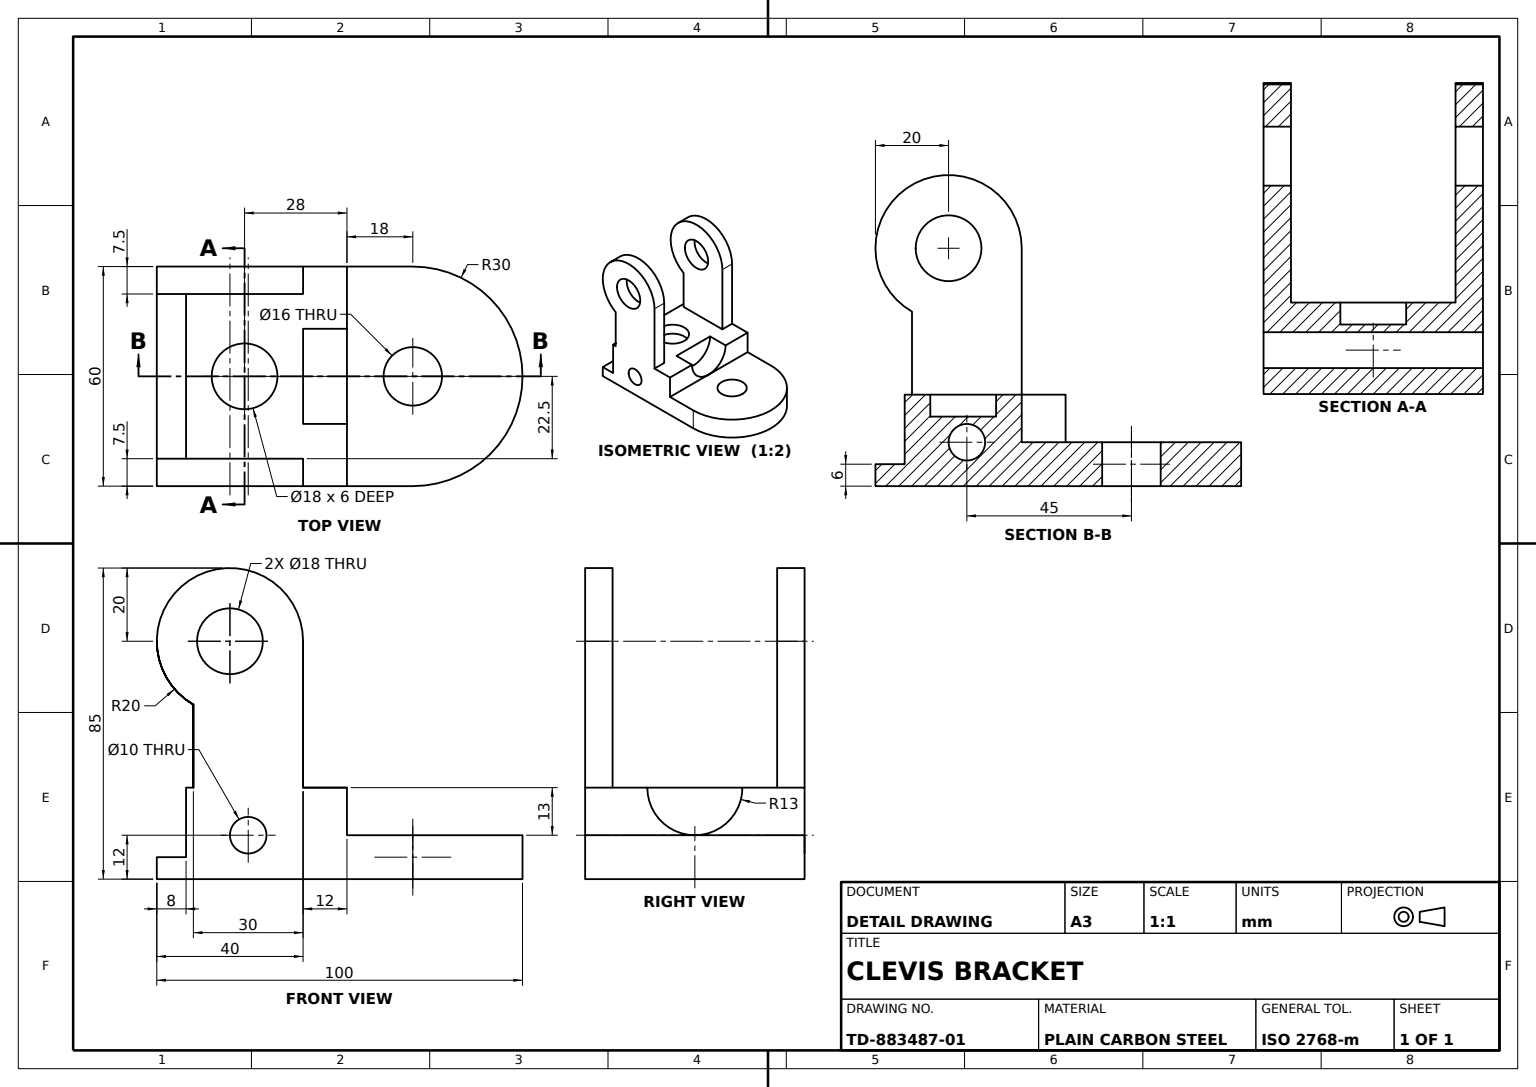
SolidWorks part; units mm, degrees
material "Plain Carbon Steel"
ref_plane "Front Plane" through (0, 0, 0) normal (0, 0, 1) x (1, 0, 0)
ref_plane "Top Plane" through (0, 0, 0) normal (0, 1, 0) x (1, 0, 0)
ref_plane "Right Plane" through (0, 0, 0) normal (1, 0, 0) x (0, 0, -1)
sketch "Base Plate Sketch" plane through (0, 0, 0) normal (0, 1, 0) x (1, 0, 0)
  line L0 (0, -103.791) -> (0, 103.791) construction
  line L1 (-133.486, 0) -> (133.486, 0) construction
  line L2 (30, 0) -> (30, -70)
  line L3 (30, -70) -> (-30, -70)
  line L4 (-30, -70) -> (-30, 0)
  arc A0 (30, 0) -> (-30, 0) centre (0, 0) ccw
  point P4 (0, 0)
  point P8 (0, 0)
  dimension "D1" = 60
  dimension "D2" = 70
extrude "Base Plate" add sketch "Base Plate Sketch" along normal blind 12
sketch "Centre Hole Ø16 Sketch" plane through (0, 12, 0) normal (0, 1, 0) x (1, 0, 0)
  circle A0 centre (0, 0) radius 8
  dimension "D1" = 16
extrude "Centre Hole Ø16" cut sketch "Centre Hole Ø16 Sketch" against normal blind 12
sketch "Groove Sketch" plane through (0, 12, 0) normal (0, 1, 0) x (1, 0, 0)
  line L0 (-30, -70) -> (30, -70)
  line L1 (30, -70) -> (30, -62)
  line L2 (30, -70) -> (30, 0) construction
  line L3 (30, -62) -> (-30, -62)
  line L4 (-30, 0) -> (-30, -70) construction
  line L5 (-30, -62) -> (-30, -70)
  dimension "D1" = 8
extrude "Groove 8mm" cut sketch "Groove Sketch" against normal blind 6
sketch "Upright Wall Sketch" plane through (30, 0, 0) normal (1, 0, 0) x (0, 0, -1)
  line L0 (-18, 12) -> (-18, 25)
  line L1 (-30, 25) -> (-62, 25)
  line L2 (-18, 25) -> (-30, 25)
  line L3 (-62, 12) -> (0, 12) construction
  line L4 (-30, 25) -> (-30, 65)
  line L6 (-62, 12) -> (-62, 49)
  arc A0 (-30, 65) -> (-62, 49) centre (-50, 65) ccw
  arc A1 (-30, 65) -> (-62, 49) centre (-50, 65) ccw
  circle A2 centre (-50, 65) radius 9
  line M10 (0, 12) -> (-62, 12)
  dimension "D5" = 40
  dimension "D6" = 18
  dimension "D1" = 13
  dimension "D2" = 12
  dimension "D3" = 40
  dimension "D4" = 18
extrude "Upright Wall" add sketch "Upright Wall Sketch" against normal blind 60 contours L6 L0 L2 L1 M10
sketch "Pin Lug Sketch" plane through (30, 0, 0) normal (1, 0, 0) x (0, 0, -1)
  line L0 (-30, 25) -> (-30, 65)
  line L1 (-18, 25) -> (-30, 25)
  line L2 (-60, 25) -> (-60, 47.6795)
  line L3 (-30, 25) -> (-60, 25)
  arc A1 (-30, 65) -> (-60, 47.6795) centre (-50, 65) ccw
  circle A2 centre (-50, 65) radius 9
  dimension "D3" = 40
  dimension "D4" = 30
  dimension "D5" = 18
  dimension "D1" = 40
  dimension "D2" = 12
extrude "Pin Lug" add sketch "Pin Lug Sketch" against normal blind 7.5
mirror "Pin Lug Mirror" about plane through (0, 0, 0) normal (1, 0, 0) of "Pin Lug"
sketch "Hole Ø26 Sketch" plane through (0, 0, 18) normal (0, 0, -1) x (-1, 0, 0)
  line L0 (30, 25) -> (-30, 25) construction
  circle A0 centre (0, 25) radius 13
  dimension "D1" = 26
extrude "Hole Ø26" cut sketch "Hole Ø26 Sketch" against normal blind 12
sketch "Recess Ø18 Sketch" plane through (0, 25, 0) normal (0, 1, 0) x (1, 0, 0)
  line L0 (-30, -18) -> (-30, -30) construction
  circle A1 centre (0, -46) radius 9
  dimension "D1" = 18
  dimension "D2" = 30
  dimension "D3" = 28
extrude "Recess Ø18" cut sketch "Recess Ø18 Sketch" against normal blind 6
sketch "Side Hole Ø10 Sketch" plane through (30, 0, 0) normal (1, 0, 0) x (0, 0, -1)
  circle A0 centre (-45, 12) radius 5
  dimension "D2" = 45
  dimension "D1" = 10
  dimension "D3" = 12
extrude "Side Hole Ø10" cut sketch "Side Hole Ø10 Sketch" against normal blind 13
sketch "Lug Pin Hole Ø10 Sketch" plane through (-30, 0, 0) normal (-1, 0, 0) x (0, 0, 1)
  line L0 (62, 6) -> (70, 6) construction
  line L1 (30, 25) -> (30, 65) construction
  circle A0 centre (45, 12) radius 5
  dimension "D3" = 10
  dimension "D1" = 15
  dimension "D2" = 6
extrude "Lug Pin Hole Ø10" cut sketch "Lug Pin Hole Ø10 Sketch" against normal blind 85
